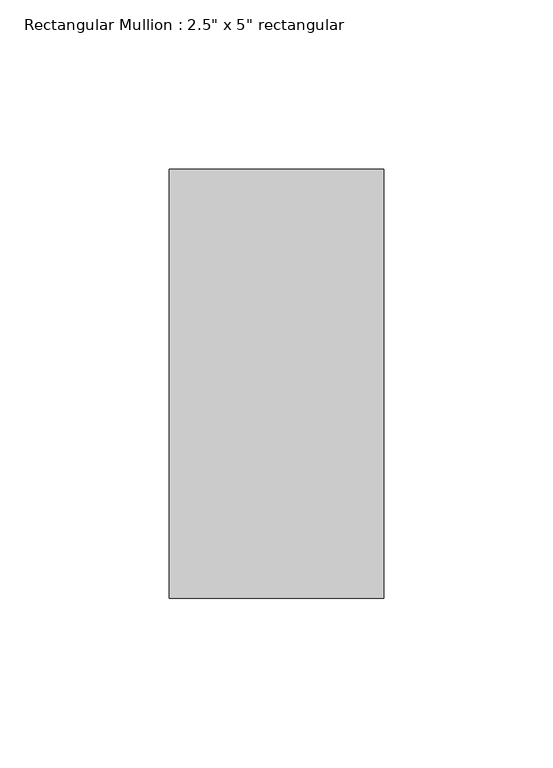
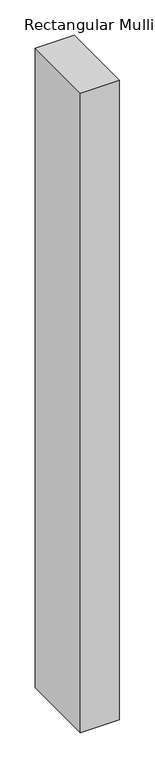
"""IFC4 building model written with IfcOpenShell, lengths in millimetres: member geometry."""

from ifc_helpers import new_model, si_unit, frame, origin, place, context, project, spatial, polyline, outline, extrude, source, transform, mapped, element, save


def member_d518c94e(model_context):
    return source(origin(), model_context, "Body", "SweptSolid", [
        extrude(outline(polyline([(31.75, 63.5), (31.75, -63.5), (-31.75, -63.5), (-31.75, 63.5), (31.75, 63.5)])), frame((0.0, 0.0, -1101.9692307), z_axis=(0.0, 0.0, 1.0), x_axis=(1.0, 0.0, 0.0)), (0.0, 0.0, 1.0), 1101.9692307),
    ])


if __name__ == "__main__":
    model = new_model("IFC4")
    model_context = context("Model", 3, world=origin())
    ifc_project = project(units=[si_unit("LENGTHUNIT", "METRE", prefix="MILLI")], contexts=[model_context])
    site = spatial("IfcSite", under=ifc_project)
    building = spatial("IfcBuilding", under=site)
    placement = place(None, origin())
    member_shape = member_d518c94e(model_context)
    element("IfcMember", 1, ObjectType="Rectangular Mullion : 2.5\" x 5\" rectangular", at=placement, inside=building, context=model_context, shape_type="MappedRepresentation", body=[
        mapped(member_shape, transform((0.0, 0.0, 0.0), x_axis=(1.0, 0.0, 0.0), y_axis=(0.0, 1.0, 0.0), z_axis=(0.0, 0.0, 1.0))),
    ])
    save(model, "model.ifc")

# Revit data of these elements
# Type "Rectangular Mullion : 2.5\" x 5\" rectangular"
#   built-in parameter 1007304 = 0.416667 (stored number, unit not read)
#   built-in parameter 1007301 = 0.104167 (stored number, unit not read)
#   built-in parameter 1007300 = 0.104167 (stored number, unit not read)
# Element 1 (IfcMember, "Rectangular Mullion : 2.5\" x 5\" rectangular")
#   Materials on its faces: "Aluminum"
# Materials
#   "Aluminum": class "Metal", colour RGB 247 247 247, transparency 0, Description = "Aluminum 6061", Cost = 0
